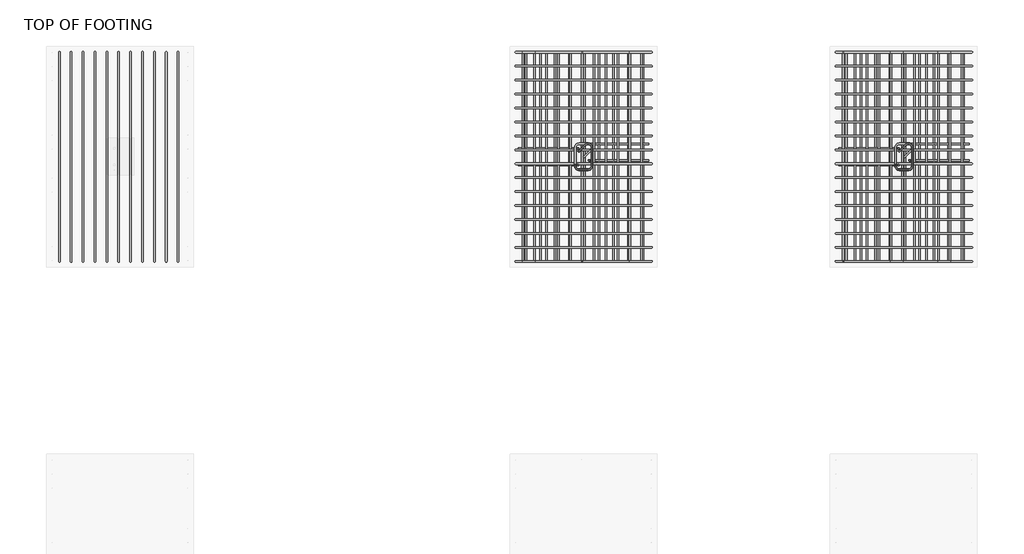
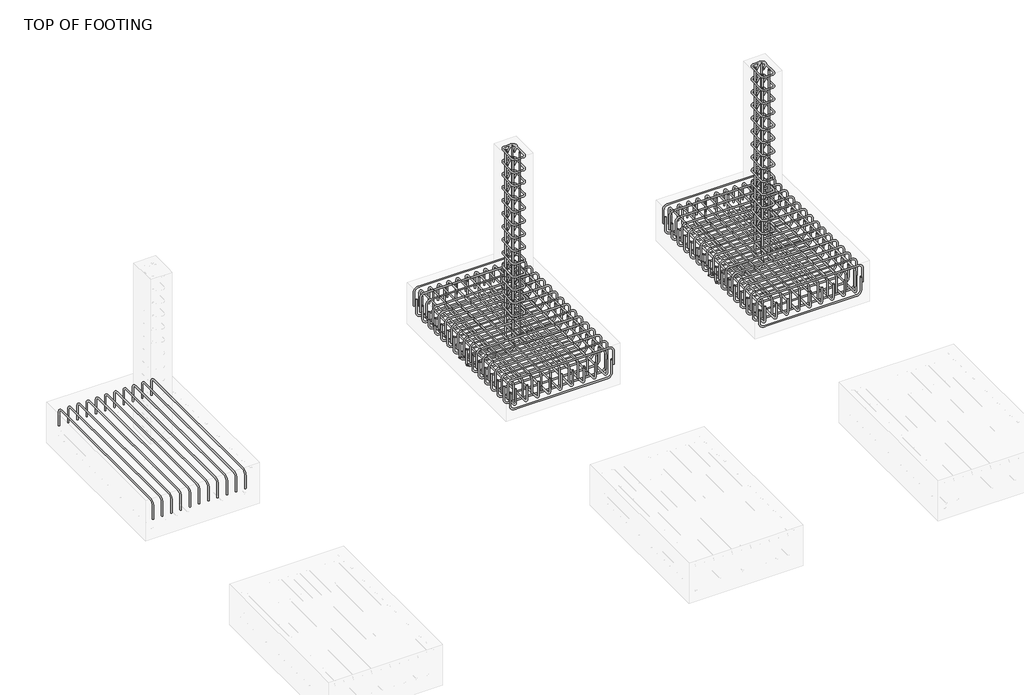
# One storey, part 8 of 8: 15 reinforcing bars.
"""IFC4 building model written with IfcOpenShell, lengths in millimetres."""

from ifc_helpers import new_model, si_unit, point, frame, origin, place, context, project, spatial, polyline, circle_curve, trimmed, segment, composite_curve, source, transform, mapped, element, save
from ifc_brep_helpers import swept_disk

model = new_model("IFC4")

# Units and contexts
model_context = context("Model", 3, world=origin())
ifc_project = project(units=[si_unit("LENGTHUNIT", "METRE", prefix="MILLI")], contexts=[model_context])

# Site, building, storey
site = spatial("IfcSite", under=ifc_project)
building = spatial("IfcBuilding", under=site)
storey = spatial("IfcBuildingStorey", under=building, Name="TOP OF FOOTING", Elevation=-1828.8)

# Reinforcing bars
placement = place(None, origin())
reinforcing_bar_shape = source(origin(), model_context, "Body", "SolidModel", [
    swept_disk(composite_curve([segment(polyline([(6846.0817577, 8966.4007933, -46.35), (6901.8253207, 9022.1443562, -46.35)]), True, "CONTINUOUS"), segment(trimmed(circle_curve(frame((6923.9931183, 8999.9765586, -46.35), z_axis=(0.0, 0.0, -1.0), x_axis=(-22.167797600000085, 22.167797600000995, 0.0)), 31.35), [point((6901.8253207, 9022.1443562, -46.35))], [point((6955.3431183, 8999.9765586, -46.35))], True, "CARTESIAN"), True, "CONTINUOUS"), segment(polyline([(6955.3431183, 8999.9765586, -46.35), (6955.3431183, 8850.5765586, -46.35)]), True, "CONTINUOUS"), segment(trimmed(circle_curve(frame((6923.9931183, 8850.5765586, -46.35), z_axis=(0.0, 0.0, -1.0), x_axis=(31.350000000000364, 0.0, 0.0)), 31.35), [point((6955.3431183, 8850.5765586, -46.35))], [point((6923.9931183, 8819.2265586, -46.35))], True, "CARTESIAN"), True, "CONTINUOUS"), segment(polyline([(6923.9931183, 8819.2265586, -46.35), (6850.7931183, 8819.2265586, -46.35)]), True, "CONTINUOUS"), segment(trimmed(circle_curve(frame((6850.7931183, 8850.5205096, -44.4761991), z_axis=(0.0, 0.05977036468717588, -0.9982121535551258), x_axis=(0.0, -31.29395100000147, -1.873800899999999)), 31.35), [point((6850.7931183, 8819.2265586, -46.35))], [point((6819.4431183, 8850.5205096, -44.4761991))], True, "CARTESIAN"), True, "CONTINUOUS"), segment(polyline([(6819.4431183, 8850.5205096, -44.4761991), (6819.4431183, 9000.0326076, -35.5238009)]), True, "CONTINUOUS"), segment(trimmed(circle_curve(frame((6850.7931183, 9000.0326076, -35.5238009), z_axis=(0.0, 0.05977036468717588, -0.9982121535551258), x_axis=(-31.350000000000364, 0.0, 0.0)), 31.35), [point((6819.4431183, 9000.0326076, -35.5238009))], [point((6850.7931183, 9031.3265586, -33.65))], True, "CARTESIAN"), True, "CONTINUOUS"), segment(polyline([(6850.7931183, 9031.3265586, -33.65), (6923.9931183, 9031.3265586, -33.65)]), True, "CONTINUOUS"), segment(trimmed(circle_curve(frame((6923.9931183, 8999.9765586, -33.65), z_axis=(0.0, 0.0, -1.0), x_axis=(0.0, 31.350000000000364, 0.0)), 31.35), [point((6923.9931183, 9031.3265586, -33.65))], [point((6946.1609159, 8977.808761, -33.65))], True, "CARTESIAN"), True, "CONTINUOUS"), segment(polyline([(6946.1609159, 8977.808761, -33.65), (6890.4173529, 8922.0651981, -33.65)]), True, "CONTINUOUS")], self_intersect=False), 6.35),
])
element("IfcReinforcingBar", 1, at=placement, inside=storey, context=model_context, shape_type="MappedRepresentation", body=[
    mapped(reinforcing_bar_shape, transform((0.0, 0.0, 0.0), x_axis=(1.0, 0.0, 0.0), y_axis=(0.0, 1.0, 0.0), z_axis=(0.0, 0.0, 1.0))),
    mapped(reinforcing_bar_shape, transform((0.0, 0.0, -144.675), x_axis=(1.0, 0.0, 0.0), y_axis=(0.0, 1.0, 0.0), z_axis=(0.0, 0.0, 1.0))),
    mapped(reinforcing_bar_shape, transform((0.0, 0.0, -289.35), x_axis=(1.0, 0.0, 0.0), y_axis=(0.0, 1.0, 0.0), z_axis=(0.0, 0.0, 1.0))),
    mapped(reinforcing_bar_shape, transform((0.0, 0.0, -434.025), x_axis=(1.0, 0.0, 0.0), y_axis=(0.0, 1.0, 0.0), z_axis=(0.0, 0.0, 1.0))),
    mapped(reinforcing_bar_shape, transform((0.0, 0.0, -578.7), x_axis=(1.0, 0.0, 0.0), y_axis=(0.0, 1.0, 0.0), z_axis=(0.0, 0.0, 1.0))),
    mapped(reinforcing_bar_shape, transform((0.0, 0.0, -723.375), x_axis=(1.0, 0.0, 0.0), y_axis=(0.0, 1.0, 0.0), z_axis=(0.0, 0.0, 1.0))),
    mapped(reinforcing_bar_shape, transform((0.0, 0.0, -868.05), x_axis=(1.0, 0.0, 0.0), y_axis=(0.0, 1.0, 0.0), z_axis=(0.0, 0.0, 1.0))),
    mapped(reinforcing_bar_shape, transform((0.0, 0.0, -1012.725), x_axis=(1.0, 0.0, 0.0), y_axis=(0.0, 1.0, 0.0), z_axis=(0.0, 0.0, 1.0))),
    mapped(reinforcing_bar_shape, transform((0.0, 0.0, -1157.4), x_axis=(1.0, 0.0, 0.0), y_axis=(0.0, 1.0, 0.0), z_axis=(0.0, 0.0, 1.0))),
    mapped(reinforcing_bar_shape, transform((0.0, 0.0, -1302.075), x_axis=(1.0, 0.0, 0.0), y_axis=(0.0, 1.0, 0.0), z_axis=(0.0, 0.0, 1.0))),
    mapped(reinforcing_bar_shape, transform((0.0, 0.0, -1446.75), x_axis=(1.0, 0.0, 0.0), y_axis=(0.0, 1.0, 0.0), z_axis=(0.0, 0.0, 1.0))),
    mapped(reinforcing_bar_shape, transform((0.0, 0.0, -1591.425), x_axis=(1.0, 0.0, 0.0), y_axis=(0.0, 1.0, 0.0), z_axis=(0.0, 0.0, 1.0))),
    mapped(reinforcing_bar_shape, transform((0.0, 0.0, -1736.1), x_axis=(1.0, 0.0, 0.0), y_axis=(0.0, 1.0, 0.0), z_axis=(0.0, 0.0, 1.0))),
])
reinforcing_bar_2_shape = source(origin(), model_context, "Body", "SolidModel", [
    swept_disk(composite_curve([segment(polyline([(7420.419602, 8895.4265586, -2177.1384798), (6979.2627797, 8895.4265586, -2177.1384798)]), True, "CONTINUOUS"), segment(trimmed(circle_curve(frame((6979.2627797, 8895.4265586, -2130.7884798), z_axis=(0.0, 1.0, 0.0), x_axis=(0.0, 0.0, -46.34999999999991)), 46.35), [point((6979.2627797, 8895.4265586, -2177.1384798))], [point((6932.9127797, 8895.4265586, -2130.7884798))], True, "CARTESIAN"), True, "CONTINUOUS"), segment(polyline([(6932.9127797, 8895.4265586, -2130.7884798), (6932.9127797, 8895.4265586, -40.0)]), True, "CONTINUOUS")], self_intersect=False), 6.35),
])
element("IfcReinforcingBar", 2, at=placement, inside=storey, context=model_context, shape_type="MappedRepresentation", body=[
    mapped(reinforcing_bar_2_shape, transform((0.0, 0.0, 0.0), x_axis=(1.0, 0.0, 0.0), y_axis=(0.0, 1.0, 0.0), z_axis=(0.0, 0.0, 1.0))),
    mapped(reinforcing_bar_2_shape, transform((0.0, 135.9, 0.0), x_axis=(1.0, 0.0, 0.0), y_axis=(0.0, 1.0, 0.0), z_axis=(0.0, 0.0, 1.0))),
])
reinforcing_bar_3_shape = source(origin(), model_context, "Body", "SolidModel", [
    swept_disk(composite_curve([segment(polyline([(6354.3666346, 8857.3265586, -2177.1384798), (6795.5234568, 8857.3265586, -2177.1384798)]), True, "CONTINUOUS"), segment(trimmed(circle_curve(frame((6795.5234568, 8857.3265586, -2130.7884798), z_axis=(0.0, -1.0, 0.0), x_axis=(0.0, 0.0, -46.34999999999991)), 46.35), [point((6795.5234568, 8857.3265586, -2177.1384798))], [point((6841.8734568, 8857.3265586, -2130.7884798))], True, "CARTESIAN"), True, "CONTINUOUS"), segment(polyline([(6841.8734568, 8857.3265586, -2130.7884798), (6841.8734568, 8857.3265586, -40.0)]), True, "CONTINUOUS")], self_intersect=False), 6.35),
])
element("IfcReinforcingBar", 3, at=placement, inside=storey, context=model_context, shape_type="MappedRepresentation", body=[
    mapped(reinforcing_bar_3_shape, transform((0.0, 0.0, 0.0), x_axis=(1.0, 0.0, 0.0), y_axis=(0.0, 1.0, 0.0), z_axis=(0.0, 0.0, 1.0))),
    mapped(reinforcing_bar_3_shape, transform((0.0, 135.9, 0.0), x_axis=(1.0, 0.0, 0.0), y_axis=(0.0, 1.0, 0.0), z_axis=(0.0, 0.0, 1.0))),
])
reinforcing_bar_4_shape = source(origin(), model_context, "Body", "SolidModel", [
    swept_disk(composite_curve([segment(polyline([(9462.2817577, 8966.4007933, -46.35), (9518.0253207, 9022.1443562, -46.35)]), True, "CONTINUOUS"), segment(trimmed(circle_curve(frame((9540.1931183, 8999.9765586, -46.35), z_axis=(0.0, 0.0, -1.0), x_axis=(-22.167797599999176, 22.167797600000995, 0.0)), 31.35), [point((9518.0253207, 9022.1443562, -46.35))], [point((9571.5431183, 8999.9765586, -46.35))], True, "CARTESIAN"), True, "CONTINUOUS"), segment(polyline([(9571.5431183, 8999.9765586, -46.35), (9571.5431183, 8850.5765586, -46.35)]), True, "CONTINUOUS"), segment(trimmed(circle_curve(frame((9540.1931183, 8850.5765586, -46.35), z_axis=(0.0, 0.0, -1.0), x_axis=(31.350000000000364, 0.0, 0.0)), 31.35), [point((9571.5431183, 8850.5765586, -46.35))], [point((9540.1931183, 8819.2265586, -46.35))], True, "CARTESIAN"), True, "CONTINUOUS"), segment(polyline([(9540.1931183, 8819.2265586, -46.35), (9466.9931183, 8819.2265586, -46.35)]), True, "CONTINUOUS"), segment(trimmed(circle_curve(frame((9466.9931183, 8850.5205096, -44.4761991), z_axis=(0.0, 0.05977036468717588, -0.9982121535551258), x_axis=(0.0, -31.29395100000147, -1.873800899999999)), 31.35), [point((9466.9931183, 8819.2265586, -46.35))], [point((9435.6431183, 8850.5205096, -44.4761991))], True, "CARTESIAN"), True, "CONTINUOUS"), segment(polyline([(9435.6431183, 8850.5205096, -44.4761991), (9435.6431183, 9000.0326076, -35.5238009)]), True, "CONTINUOUS"), segment(trimmed(circle_curve(frame((9466.9931183, 9000.0326076, -35.5238009), z_axis=(0.0, 0.05977036468717588, -0.9982121535551258), x_axis=(-31.350000000000364, 0.0, 0.0)), 31.35), [point((9435.6431183, 9000.0326076, -35.5238009))], [point((9466.9931183, 9031.3265586, -33.65))], True, "CARTESIAN"), True, "CONTINUOUS"), segment(polyline([(9466.9931183, 9031.3265586, -33.65), (9540.1931183, 9031.3265586, -33.65)]), True, "CONTINUOUS"), segment(trimmed(circle_curve(frame((9540.1931183, 8999.9765586, -33.65), z_axis=(0.0, 0.0, -1.0), x_axis=(0.0, 31.350000000000364, 0.0)), 31.35), [point((9540.1931183, 9031.3265586, -33.65))], [point((9562.3609159, 8977.808761, -33.65))], True, "CARTESIAN"), True, "CONTINUOUS"), segment(polyline([(9562.3609159, 8977.808761, -33.65), (9506.6173529, 8922.0651981, -33.65)]), True, "CONTINUOUS")], self_intersect=False), 6.35),
])
element("IfcReinforcingBar", 4, at=placement, inside=storey, context=model_context, shape_type="MappedRepresentation", body=[
    mapped(reinforcing_bar_4_shape, transform((0.0, 0.0, 0.0), x_axis=(1.0, 0.0, 0.0), y_axis=(0.0, 1.0, 0.0), z_axis=(0.0, 0.0, 1.0))),
    mapped(reinforcing_bar_4_shape, transform((0.0, 0.0, -144.675), x_axis=(1.0, 0.0, 0.0), y_axis=(0.0, 1.0, 0.0), z_axis=(0.0, 0.0, 1.0))),
    mapped(reinforcing_bar_4_shape, transform((0.0, 0.0, -289.35), x_axis=(1.0, 0.0, 0.0), y_axis=(0.0, 1.0, 0.0), z_axis=(0.0, 0.0, 1.0))),
    mapped(reinforcing_bar_4_shape, transform((0.0, 0.0, -434.025), x_axis=(1.0, 0.0, 0.0), y_axis=(0.0, 1.0, 0.0), z_axis=(0.0, 0.0, 1.0))),
    mapped(reinforcing_bar_4_shape, transform((0.0, 0.0, -578.7), x_axis=(1.0, 0.0, 0.0), y_axis=(0.0, 1.0, 0.0), z_axis=(0.0, 0.0, 1.0))),
    mapped(reinforcing_bar_4_shape, transform((0.0, 0.0, -723.375), x_axis=(1.0, 0.0, 0.0), y_axis=(0.0, 1.0, 0.0), z_axis=(0.0, 0.0, 1.0))),
    mapped(reinforcing_bar_4_shape, transform((0.0, 0.0, -868.05), x_axis=(1.0, 0.0, 0.0), y_axis=(0.0, 1.0, 0.0), z_axis=(0.0, 0.0, 1.0))),
    mapped(reinforcing_bar_4_shape, transform((0.0, 0.0, -1012.725), x_axis=(1.0, 0.0, 0.0), y_axis=(0.0, 1.0, 0.0), z_axis=(0.0, 0.0, 1.0))),
    mapped(reinforcing_bar_4_shape, transform((0.0, 0.0, -1157.4), x_axis=(1.0, 0.0, 0.0), y_axis=(0.0, 1.0, 0.0), z_axis=(0.0, 0.0, 1.0))),
    mapped(reinforcing_bar_4_shape, transform((0.0, 0.0, -1302.075), x_axis=(1.0, 0.0, 0.0), y_axis=(0.0, 1.0, 0.0), z_axis=(0.0, 0.0, 1.0))),
    mapped(reinforcing_bar_4_shape, transform((0.0, 0.0, -1446.75), x_axis=(1.0, 0.0, 0.0), y_axis=(0.0, 1.0, 0.0), z_axis=(0.0, 0.0, 1.0))),
    mapped(reinforcing_bar_4_shape, transform((0.0, 0.0, -1591.425), x_axis=(1.0, 0.0, 0.0), y_axis=(0.0, 1.0, 0.0), z_axis=(0.0, 0.0, 1.0))),
    mapped(reinforcing_bar_4_shape, transform((0.0, 0.0, -1736.1), x_axis=(1.0, 0.0, 0.0), y_axis=(0.0, 1.0, 0.0), z_axis=(0.0, 0.0, 1.0))),
])
reinforcing_bar_5_shape = source(origin(), model_context, "Body", "SolidModel", [
    swept_disk(composite_curve([segment(polyline([(10036.619602, 8895.4265586, -2177.1384798), (9595.4627797, 8895.4265586, -2177.1384798)]), True, "CONTINUOUS"), segment(trimmed(circle_curve(frame((9595.4627797, 8895.4265586, -2130.7884798), z_axis=(0.0, 1.0, 0.0), x_axis=(0.0, 0.0, -46.34999999999991)), 46.35), [point((9595.4627797, 8895.4265586, -2177.1384798))], [point((9549.1127797, 8895.4265586, -2130.7884798))], True, "CARTESIAN"), True, "CONTINUOUS"), segment(polyline([(9549.1127797, 8895.4265586, -2130.7884798), (9549.1127797, 8895.4265586, -40.0)]), True, "CONTINUOUS")], self_intersect=False), 6.35),
])
element("IfcReinforcingBar", 5, at=placement, inside=storey, context=model_context, shape_type="MappedRepresentation", body=[
    mapped(reinforcing_bar_5_shape, transform((0.0, 0.0, 0.0), x_axis=(1.0, 0.0, 0.0), y_axis=(0.0, 1.0, 0.0), z_axis=(0.0, 0.0, 1.0))),
    mapped(reinforcing_bar_5_shape, transform((0.0, 135.9, 0.0), x_axis=(1.0, 0.0, 0.0), y_axis=(0.0, 1.0, 0.0), z_axis=(0.0, 0.0, 1.0))),
])
reinforcing_bar_6_shape = source(origin(), model_context, "Body", "SolidModel", [
    swept_disk(composite_curve([segment(polyline([(8970.5666346, 8857.3265586, -2177.1384798), (9411.7234568, 8857.3265586, -2177.1384798)]), True, "CONTINUOUS"), segment(trimmed(circle_curve(frame((9411.7234568, 8857.3265586, -2130.7884798), z_axis=(0.0, -1.0, 0.0), x_axis=(0.0, 0.0, -46.34999999999991)), 46.35), [point((9411.7234568, 8857.3265586, -2177.1384798))], [point((9458.0734568, 8857.3265586, -2130.7884798))], True, "CARTESIAN"), True, "CONTINUOUS"), segment(polyline([(9458.0734568, 8857.3265586, -2130.7884798), (9458.0734568, 8857.3265586, -40.0)]), True, "CONTINUOUS")], self_intersect=False), 6.35),
])
element("IfcReinforcingBar", 6, at=placement, inside=storey, context=model_context, shape_type="MappedRepresentation", body=[
    mapped(reinforcing_bar_6_shape, transform((0.0, 0.0, 0.0), x_axis=(1.0, 0.0, 0.0), y_axis=(0.0, 1.0, 0.0), z_axis=(0.0, 0.0, 1.0))),
    mapped(reinforcing_bar_6_shape, transform((0.0, 135.9, 0.0), x_axis=(1.0, 0.0, 0.0), y_axis=(0.0, 1.0, 0.0), z_axis=(0.0, 0.0, 1.0))),
])
reinforcing_bar_7_shape = source(origin(), model_context, "Body", "SolidModel", [
    swept_disk(composite_curve([segment(polyline([(3577.1331701, 9778.9265586, -2094.8977257), (3577.1331701, 9778.9265586, -1947.5977257)]), True, "CONTINUOUS"), segment(trimmed(circle_curve(frame((3577.1331701, 9732.5765586, -1947.5977257), z_axis=(1.0, 0.0, 0.0), x_axis=(0.0, 46.350000000000364, 0.0)), 46.35), [point((3577.1331701, 9778.9265586, -1947.5977257))], [point((3577.1331701, 9732.5765586, -1901.2477257))], True, "CARTESIAN"), True, "CONTINUOUS"), segment(polyline([(3577.1331701, 9732.5765586, -1901.2477257), (3577.1331701, 8117.9765586, -1901.2477257)]), True, "CONTINUOUS"), segment(trimmed(circle_curve(frame((3577.1331701, 8117.9765586, -1947.5977257), z_axis=(1.0, 0.0, 0.0), x_axis=(0.0, 0.0, 46.34999999999991)), 46.35), [point((3577.1331701, 8117.9765586, -1901.2477257))], [point((3577.1331701, 8071.6265586, -1947.5977257))], True, "CARTESIAN"), True, "CONTINUOUS"), segment(polyline([(3577.1331701, 8071.6265586, -1947.5977257), (3577.1331701, 8071.6265586, -2094.8977257)]), True, "CONTINUOUS")], self_intersect=False), 6.35),
])
element("IfcReinforcingBar", 7, at=placement, inside=storey, context=model_context, shape_type="MappedRepresentation", body=[
    mapped(reinforcing_bar_7_shape, transform((0.0, 0.0, 0.0), x_axis=(1.0, 0.0, 0.0), y_axis=(0.0, 1.0, 0.0), z_axis=(0.0, 0.0, 1.0))),
    mapped(reinforcing_bar_7_shape, transform((-97.0050815, 0.0, 0.0), x_axis=(1.0, 0.0, 0.0), y_axis=(0.0, 1.0, 0.0), z_axis=(0.0, 0.0, 1.0))),
    mapped(reinforcing_bar_7_shape, transform((-194.0101631, 0.0, 0.0), x_axis=(1.0, 0.0, 0.0), y_axis=(0.0, 1.0, 0.0), z_axis=(0.0, 0.0, 1.0))),
    mapped(reinforcing_bar_7_shape, transform((-291.0152446, 0.0, 0.0), x_axis=(1.0, 0.0, 0.0), y_axis=(0.0, 1.0, 0.0), z_axis=(0.0, 0.0, 1.0))),
    mapped(reinforcing_bar_7_shape, transform((-388.0203261, 0.0, 0.0), x_axis=(1.0, 0.0, 0.0), y_axis=(0.0, 1.0, 0.0), z_axis=(0.0, 0.0, 1.0))),
    mapped(reinforcing_bar_7_shape, transform((-485.0254076, 0.0, 0.0), x_axis=(1.0, 0.0, 0.0), y_axis=(0.0, 1.0, 0.0), z_axis=(0.0, 0.0, 1.0))),
    mapped(reinforcing_bar_7_shape, transform((-582.0304892, 0.0, 0.0), x_axis=(1.0, 0.0, 0.0), y_axis=(0.0, 1.0, 0.0), z_axis=(0.0, 0.0, 1.0))),
    mapped(reinforcing_bar_7_shape, transform((-679.0355707, 0.0, 0.0), x_axis=(1.0, 0.0, 0.0), y_axis=(0.0, 1.0, 0.0), z_axis=(0.0, 0.0, 1.0))),
    mapped(reinforcing_bar_7_shape, transform((-776.0406522, 0.0, 0.0), x_axis=(1.0, 0.0, 0.0), y_axis=(0.0, 1.0, 0.0), z_axis=(0.0, 0.0, 1.0))),
    mapped(reinforcing_bar_7_shape, transform((-873.0457338, 0.0, 0.0), x_axis=(1.0, 0.0, 0.0), y_axis=(0.0, 1.0, 0.0), z_axis=(0.0, 0.0, 1.0))),
    mapped(reinforcing_bar_7_shape, transform((-970.0508153, 0.0, 0.0), x_axis=(1.0, 0.0, 0.0), y_axis=(0.0, 1.0, 0.0), z_axis=(0.0, 0.0, 1.0))),
])
reinforcing_bar_8_shape = source(origin(), model_context, "Body", "SolidModel", [
    swept_disk(composite_curve([segment(polyline([(7421.6426771, 9778.9265586, -2008.2544267), (7421.6426771, 9778.9265586, -2155.5544267)]), True, "CONTINUOUS"), segment(trimmed(circle_curve(frame((7375.2926771, 9778.9265586, -2155.5544267), z_axis=(0.0, 1.0, 0.0), x_axis=(46.349999999999454, 0.0, 0.0)), 46.35), [point((7421.6426771, 9778.9265586, -2155.5544267))], [point((7375.2926771, 9778.9265586, -2201.9044267))], True, "CARTESIAN"), True, "CONTINUOUS"), segment(polyline([(7375.2926771, 9778.9265586, -2201.9044267), (6404.2766408, 9778.9265586, -2201.9044267)]), True, "CONTINUOUS"), segment(trimmed(circle_curve(frame((6404.2766408, 9778.9265586, -2155.5544267), z_axis=(0.0, 1.0, 0.0), x_axis=(0.0, 0.0, -46.34999999999991)), 46.35), [point((6404.2766408, 9778.9265586, -2201.9044267))], [point((6357.9266408, 9778.9265586, -2155.5544267))], True, "CARTESIAN"), True, "CONTINUOUS"), segment(polyline([(6357.9266408, 9778.9265586, -2155.5544267), (6357.9266408, 9778.9265586, -2008.2544267)]), True, "CONTINUOUS")], self_intersect=False), 6.35),
])
element("IfcReinforcingBar", 8, at=placement, inside=storey, context=model_context, shape_type="MappedRepresentation", body=[
    mapped(reinforcing_bar_8_shape, transform((0.0, 0.0, 0.0), x_axis=(1.0, 0.0, 0.0), y_axis=(0.0, 1.0, 0.0), z_axis=(0.0, 0.0, 1.0))),
    mapped(reinforcing_bar_8_shape, transform((0.0, -113.82, 0.0), x_axis=(1.0, 0.0, 0.0), y_axis=(0.0, 1.0, 0.0), z_axis=(0.0, 0.0, 1.0))),
    mapped(reinforcing_bar_8_shape, transform((0.0, -227.64, 0.0), x_axis=(1.0, 0.0, 0.0), y_axis=(0.0, 1.0, 0.0), z_axis=(0.0, 0.0, 1.0))),
    mapped(reinforcing_bar_8_shape, transform((0.0, -341.46, 0.0), x_axis=(1.0, 0.0, 0.0), y_axis=(0.0, 1.0, 0.0), z_axis=(0.0, 0.0, 1.0))),
    mapped(reinforcing_bar_8_shape, transform((0.0, -455.28, 0.0), x_axis=(1.0, 0.0, 0.0), y_axis=(0.0, 1.0, 0.0), z_axis=(0.0, 0.0, 1.0))),
    mapped(reinforcing_bar_8_shape, transform((0.0, -569.1, 0.0), x_axis=(1.0, 0.0, 0.0), y_axis=(0.0, 1.0, 0.0), z_axis=(0.0, 0.0, 1.0))),
    mapped(reinforcing_bar_8_shape, transform((0.0, -682.92, 0.0), x_axis=(1.0, 0.0, 0.0), y_axis=(0.0, 1.0, 0.0), z_axis=(0.0, 0.0, 1.0))),
    mapped(reinforcing_bar_8_shape, transform((0.0, -796.74, 0.0), x_axis=(1.0, 0.0, 0.0), y_axis=(0.0, 1.0, 0.0), z_axis=(0.0, 0.0, 1.0))),
    mapped(reinforcing_bar_8_shape, transform((0.0, -910.56, 0.0), x_axis=(1.0, 0.0, 0.0), y_axis=(0.0, 1.0, 0.0), z_axis=(0.0, 0.0, 1.0))),
    mapped(reinforcing_bar_8_shape, transform((0.0, -1024.38, 0.0), x_axis=(1.0, 0.0, 0.0), y_axis=(0.0, 1.0, 0.0), z_axis=(0.0, 0.0, 1.0))),
    mapped(reinforcing_bar_8_shape, transform((0.0, -1138.2, 0.0), x_axis=(1.0, 0.0, 0.0), y_axis=(0.0, 1.0, 0.0), z_axis=(0.0, 0.0, 1.0))),
    mapped(reinforcing_bar_8_shape, transform((0.0, -1252.02, 0.0), x_axis=(1.0, 0.0, 0.0), y_axis=(0.0, 1.0, 0.0), z_axis=(0.0, 0.0, 1.0))),
    mapped(reinforcing_bar_8_shape, transform((0.0, -1365.84, 0.0), x_axis=(1.0, 0.0, 0.0), y_axis=(0.0, 1.0, 0.0), z_axis=(0.0, 0.0, 1.0))),
    mapped(reinforcing_bar_8_shape, transform((0.0, -1479.66, 0.0), x_axis=(1.0, 0.0, 0.0), y_axis=(0.0, 1.0, 0.0), z_axis=(0.0, 0.0, 1.0))),
    mapped(reinforcing_bar_8_shape, transform((0.0, -1593.48, 0.0), x_axis=(1.0, 0.0, 0.0), y_axis=(0.0, 1.0, 0.0), z_axis=(0.0, 0.0, 1.0))),
    mapped(reinforcing_bar_8_shape, transform((0.0, -1707.3, 0.0), x_axis=(1.0, 0.0, 0.0), y_axis=(0.0, 1.0, 0.0), z_axis=(0.0, 0.0, 1.0))),
])
reinforcing_bar_9_shape = source(origin(), model_context, "Body", "SolidModel", [
    swept_disk(composite_curve([segment(polyline([(6333.7431183, 9778.9265586, -2068.8), (6333.7431183, 9778.9265586, -1921.5)]), True, "CONTINUOUS"), segment(trimmed(circle_curve(frame((6380.0931183, 9778.9265586, -1921.5), z_axis=(0.0, 1.0, 0.0), x_axis=(-46.350000000000364, 0.0, 0.0)), 46.35), [point((6333.7431183, 9778.9265586, -1921.5))], [point((6380.0931183, 9778.9265586, -1875.15))], True, "CARTESIAN"), True, "CONTINUOUS"), segment(polyline([(6380.0931183, 9778.9265586, -1875.15), (7394.6931183, 9778.9265586, -1875.15)]), True, "CONTINUOUS"), segment(trimmed(circle_curve(frame((7394.6931183, 9778.9265586, -1921.5), z_axis=(0.0, 1.0, 0.0), x_axis=(0.0, 0.0, 46.34999999999991)), 46.35), [point((7394.6931183, 9778.9265586, -1875.15))], [point((7441.0431183, 9778.9265586, -1921.5))], True, "CARTESIAN"), True, "CONTINUOUS"), segment(polyline([(7441.0431183, 9778.9265586, -1921.5), (7441.0431183, 9778.9265586, -2068.8)]), True, "CONTINUOUS")], self_intersect=False), 6.35),
])
element("IfcReinforcingBar", 9, at=placement, inside=storey, context=model_context, shape_type="MappedRepresentation", body=[
    mapped(reinforcing_bar_9_shape, transform((0.0, 0.0, 0.0), x_axis=(1.0, 0.0, 0.0), y_axis=(0.0, 1.0, 0.0), z_axis=(0.0, 0.0, 1.0))),
    mapped(reinforcing_bar_9_shape, transform((0.0, -113.82, 0.0), x_axis=(1.0, 0.0, 0.0), y_axis=(0.0, 1.0, 0.0), z_axis=(0.0, 0.0, 1.0))),
    mapped(reinforcing_bar_9_shape, transform((0.0, -227.64, 0.0), x_axis=(1.0, 0.0, 0.0), y_axis=(0.0, 1.0, 0.0), z_axis=(0.0, 0.0, 1.0))),
    mapped(reinforcing_bar_9_shape, transform((0.0, -341.46, 0.0), x_axis=(1.0, 0.0, 0.0), y_axis=(0.0, 1.0, 0.0), z_axis=(0.0, 0.0, 1.0))),
    mapped(reinforcing_bar_9_shape, transform((0.0, -455.28, 0.0), x_axis=(1.0, 0.0, 0.0), y_axis=(0.0, 1.0, 0.0), z_axis=(0.0, 0.0, 1.0))),
    mapped(reinforcing_bar_9_shape, transform((0.0, -569.1, 0.0), x_axis=(1.0, 0.0, 0.0), y_axis=(0.0, 1.0, 0.0), z_axis=(0.0, 0.0, 1.0))),
    mapped(reinforcing_bar_9_shape, transform((0.0, -682.92, 0.0), x_axis=(1.0, 0.0, 0.0), y_axis=(0.0, 1.0, 0.0), z_axis=(0.0, 0.0, 1.0))),
    mapped(reinforcing_bar_9_shape, transform((0.0, -796.74, 0.0), x_axis=(1.0, 0.0, 0.0), y_axis=(0.0, 1.0, 0.0), z_axis=(0.0, 0.0, 1.0))),
    mapped(reinforcing_bar_9_shape, transform((0.0, -910.56, 0.0), x_axis=(1.0, 0.0, 0.0), y_axis=(0.0, 1.0, 0.0), z_axis=(0.0, 0.0, 1.0))),
    mapped(reinforcing_bar_9_shape, transform((0.0, -1024.38, 0.0), x_axis=(1.0, 0.0, 0.0), y_axis=(0.0, 1.0, 0.0), z_axis=(0.0, 0.0, 1.0))),
    mapped(reinforcing_bar_9_shape, transform((0.0, -1138.2, 0.0), x_axis=(1.0, 0.0, 0.0), y_axis=(0.0, 1.0, 0.0), z_axis=(0.0, 0.0, 1.0))),
    mapped(reinforcing_bar_9_shape, transform((0.0, -1252.02, 0.0), x_axis=(1.0, 0.0, 0.0), y_axis=(0.0, 1.0, 0.0), z_axis=(0.0, 0.0, 1.0))),
    mapped(reinforcing_bar_9_shape, transform((0.0, -1365.84, 0.0), x_axis=(1.0, 0.0, 0.0), y_axis=(0.0, 1.0, 0.0), z_axis=(0.0, 0.0, 1.0))),
    mapped(reinforcing_bar_9_shape, transform((0.0, -1479.66, 0.0), x_axis=(1.0, 0.0, 0.0), y_axis=(0.0, 1.0, 0.0), z_axis=(0.0, 0.0, 1.0))),
    mapped(reinforcing_bar_9_shape, transform((0.0, -1593.48, 0.0), x_axis=(1.0, 0.0, 0.0), y_axis=(0.0, 1.0, 0.0), z_axis=(0.0, 0.0, 1.0))),
    mapped(reinforcing_bar_9_shape, transform((0.0, -1707.3, 0.0), x_axis=(1.0, 0.0, 0.0), y_axis=(0.0, 1.0, 0.0), z_axis=(0.0, 0.0, 1.0))),
])
reinforcing_bar_10_shape = source(origin(), model_context, "Body", "SolidModel", [
    swept_disk(composite_curve([segment(polyline([(6415.9651697, 9778.9265586, -1986.9111268), (6415.9651697, 9778.9265586, -2134.2111268)]), True, "CONTINUOUS"), segment(trimmed(circle_curve(frame((6415.9651697, 9732.5765586, -2134.2111268), z_axis=(-1.0, 0.0, 0.0), x_axis=(0.0, 46.350000000000364, 0.0)), 46.35), [point((6415.9651697, 9778.9265586, -2134.2111268))], [point((6415.9651697, 9732.5765586, -2180.5611268))], True, "CARTESIAN"), True, "CONTINUOUS"), segment(polyline([(6415.9651697, 9732.5765586, -2180.5611268), (6415.9651697, 8117.9765586, -2180.5611268)]), True, "CONTINUOUS"), segment(trimmed(circle_curve(frame((6415.9651697, 8117.9765586, -2134.2111268), z_axis=(-1.0, 0.0, 0.0), x_axis=(0.0, 0.0, -46.34999999999991)), 46.35), [point((6415.9651697, 8117.9765586, -2180.5611268))], [point((6415.9651697, 8071.6265586, -2134.2111268))], True, "CARTESIAN"), True, "CONTINUOUS"), segment(polyline([(6415.9651697, 8071.6265586, -2134.2111268), (6415.9651697, 8071.6265586, -1986.9111268)]), True, "CONTINUOUS")], self_intersect=False), 6.35),
])
element("IfcReinforcingBar", 10, at=placement, inside=storey, context=model_context, shape_type="MappedRepresentation", body=[
    mapped(reinforcing_bar_10_shape, transform((0.0, 0.0, 0.0), x_axis=(1.0, 0.0, 0.0), y_axis=(0.0, 1.0, 0.0), z_axis=(0.0, 0.0, 1.0))),
    mapped(reinforcing_bar_10_shape, transform((119.5564677, 0.0, 0.0), x_axis=(1.0, 0.0, 0.0), y_axis=(0.0, 1.0, 0.0), z_axis=(0.0, 0.0, 1.0))),
    mapped(reinforcing_bar_10_shape, transform((239.1129355, 0.0, 0.0), x_axis=(1.0, 0.0, 0.0), y_axis=(0.0, 1.0, 0.0), z_axis=(0.0, 0.0, 1.0))),
    mapped(reinforcing_bar_10_shape, transform((358.6694032, 0.0, 0.0), x_axis=(1.0, 0.0, 0.0), y_axis=(0.0, 1.0, 0.0), z_axis=(0.0, 0.0, 1.0))),
    mapped(reinforcing_bar_10_shape, transform((478.2258709, 0.0, 0.0), x_axis=(1.0, 0.0, 0.0), y_axis=(0.0, 1.0, 0.0), z_axis=(0.0, 0.0, 1.0))),
    mapped(reinforcing_bar_10_shape, transform((597.7823387, 0.0, 0.0), x_axis=(1.0, 0.0, 0.0), y_axis=(0.0, 1.0, 0.0), z_axis=(0.0, 0.0, 1.0))),
    mapped(reinforcing_bar_10_shape, transform((717.3388064, 0.0, 0.0), x_axis=(1.0, 0.0, 0.0), y_axis=(0.0, 1.0, 0.0), z_axis=(0.0, 0.0, 1.0))),
    mapped(reinforcing_bar_10_shape, transform((836.8952741, 0.0, 0.0), x_axis=(1.0, 0.0, 0.0), y_axis=(0.0, 1.0, 0.0), z_axis=(0.0, 0.0, 1.0))),
    mapped(reinforcing_bar_10_shape, transform((956.4517419, 0.0, 0.0), x_axis=(1.0, 0.0, 0.0), y_axis=(0.0, 1.0, 0.0), z_axis=(0.0, 0.0, 1.0))),
])
reinforcing_bar_11_shape = source(origin(), model_context, "Body", "SolidModel", [
    swept_disk(composite_curve([segment(polyline([(7361.7331701, 9778.9265586, -2094.8977257), (7361.7331701, 9778.9265586, -1947.5977257)]), True, "CONTINUOUS"), segment(trimmed(circle_curve(frame((7361.7331701, 9732.5765586, -1947.5977257), z_axis=(1.0, 0.0, 0.0), x_axis=(0.0, 46.350000000000364, 0.0)), 46.35), [point((7361.7331701, 9778.9265586, -1947.5977257))], [point((7361.7331701, 9732.5765586, -1901.2477257))], True, "CARTESIAN"), True, "CONTINUOUS"), segment(polyline([(7361.7331701, 9732.5765586, -1901.2477257), (7361.7331701, 8117.9765586, -1901.2477257)]), True, "CONTINUOUS"), segment(trimmed(circle_curve(frame((7361.7331701, 8117.9765586, -1947.5977257), z_axis=(1.0, 0.0, 0.0), x_axis=(0.0, 0.0, 46.34999999999991)), 46.35), [point((7361.7331701, 8117.9765586, -1901.2477257))], [point((7361.7331701, 8071.6265586, -1947.5977257))], True, "CARTESIAN"), True, "CONTINUOUS"), segment(polyline([(7361.7331701, 8071.6265586, -1947.5977257), (7361.7331701, 8071.6265586, -2094.8977257)]), True, "CONTINUOUS")], self_intersect=False), 6.35),
])
element("IfcReinforcingBar", 11, at=placement, inside=storey, context=model_context, shape_type="MappedRepresentation", body=[
    mapped(reinforcing_bar_11_shape, transform((0.0, 0.0, 0.0), x_axis=(1.0, 0.0, 0.0), y_axis=(0.0, 1.0, 0.0), z_axis=(0.0, 0.0, 1.0))),
    mapped(reinforcing_bar_11_shape, transform((-97.0050815, 0.0, 0.0), x_axis=(1.0, 0.0, 0.0), y_axis=(0.0, 1.0, 0.0), z_axis=(0.0, 0.0, 1.0))),
    mapped(reinforcing_bar_11_shape, transform((-194.0101631, 0.0, 0.0), x_axis=(1.0, 0.0, 0.0), y_axis=(0.0, 1.0, 0.0), z_axis=(0.0, 0.0, 1.0))),
    mapped(reinforcing_bar_11_shape, transform((-291.0152446, 0.0, 0.0), x_axis=(1.0, 0.0, 0.0), y_axis=(0.0, 1.0, 0.0), z_axis=(0.0, 0.0, 1.0))),
    mapped(reinforcing_bar_11_shape, transform((-388.0203261, 0.0, 0.0), x_axis=(1.0, 0.0, 0.0), y_axis=(0.0, 1.0, 0.0), z_axis=(0.0, 0.0, 1.0))),
    mapped(reinforcing_bar_11_shape, transform((-485.0254076, 0.0, 0.0), x_axis=(1.0, 0.0, 0.0), y_axis=(0.0, 1.0, 0.0), z_axis=(0.0, 0.0, 1.0))),
    mapped(reinforcing_bar_11_shape, transform((-582.0304892, 0.0, 0.0), x_axis=(1.0, 0.0, 0.0), y_axis=(0.0, 1.0, 0.0), z_axis=(0.0, 0.0, 1.0))),
    mapped(reinforcing_bar_11_shape, transform((-679.0355707, 0.0, 0.0), x_axis=(1.0, 0.0, 0.0), y_axis=(0.0, 1.0, 0.0), z_axis=(0.0, 0.0, 1.0))),
    mapped(reinforcing_bar_11_shape, transform((-776.0406522, 0.0, 0.0), x_axis=(1.0, 0.0, 0.0), y_axis=(0.0, 1.0, 0.0), z_axis=(0.0, 0.0, 1.0))),
    mapped(reinforcing_bar_11_shape, transform((-873.0457338, 0.0, 0.0), x_axis=(1.0, 0.0, 0.0), y_axis=(0.0, 1.0, 0.0), z_axis=(0.0, 0.0, 1.0))),
    mapped(reinforcing_bar_11_shape, transform((-970.0508153, 0.0, 0.0), x_axis=(1.0, 0.0, 0.0), y_axis=(0.0, 1.0, 0.0), z_axis=(0.0, 0.0, 1.0))),
])
reinforcing_bar_12_shape = source(origin(), model_context, "Body", "SolidModel", [
    swept_disk(composite_curve([segment(polyline([(10037.8426771, 9778.9265586, -2008.2544267), (10037.8426771, 9778.9265586, -2155.5544267)]), True, "CONTINUOUS"), segment(trimmed(circle_curve(frame((9991.4926771, 9778.9265586, -2155.5544267), z_axis=(0.0, 1.0, 0.0), x_axis=(46.350000000000364, 0.0, 0.0)), 46.35), [point((10037.8426771, 9778.9265586, -2155.5544267))], [point((9991.4926771, 9778.9265586, -2201.9044267))], True, "CARTESIAN"), True, "CONTINUOUS"), segment(polyline([(9991.4926771, 9778.9265586, -2201.9044267), (9020.4766408, 9778.9265586, -2201.9044267)]), True, "CONTINUOUS"), segment(trimmed(circle_curve(frame((9020.4766408, 9778.9265586, -2155.5544267), z_axis=(0.0, 1.0, 0.0), x_axis=(0.0, 0.0, -46.34999999999991)), 46.35), [point((9020.4766408, 9778.9265586, -2201.9044267))], [point((8974.1266408, 9778.9265586, -2155.5544267))], True, "CARTESIAN"), True, "CONTINUOUS"), segment(polyline([(8974.1266408, 9778.9265586, -2155.5544267), (8974.1266408, 9778.9265586, -2008.2544267)]), True, "CONTINUOUS")], self_intersect=False), 6.35),
])
element("IfcReinforcingBar", 12, at=placement, inside=storey, context=model_context, shape_type="MappedRepresentation", body=[
    mapped(reinforcing_bar_12_shape, transform((0.0, 0.0, 0.0), x_axis=(1.0, 0.0, 0.0), y_axis=(0.0, 1.0, 0.0), z_axis=(0.0, 0.0, 1.0))),
    mapped(reinforcing_bar_12_shape, transform((0.0, -113.82, 0.0), x_axis=(1.0, 0.0, 0.0), y_axis=(0.0, 1.0, 0.0), z_axis=(0.0, 0.0, 1.0))),
    mapped(reinforcing_bar_12_shape, transform((0.0, -227.64, 0.0), x_axis=(1.0, 0.0, 0.0), y_axis=(0.0, 1.0, 0.0), z_axis=(0.0, 0.0, 1.0))),
    mapped(reinforcing_bar_12_shape, transform((0.0, -341.46, 0.0), x_axis=(1.0, 0.0, 0.0), y_axis=(0.0, 1.0, 0.0), z_axis=(0.0, 0.0, 1.0))),
    mapped(reinforcing_bar_12_shape, transform((0.0, -455.28, 0.0), x_axis=(1.0, 0.0, 0.0), y_axis=(0.0, 1.0, 0.0), z_axis=(0.0, 0.0, 1.0))),
    mapped(reinforcing_bar_12_shape, transform((0.0, -569.1, 0.0), x_axis=(1.0, 0.0, 0.0), y_axis=(0.0, 1.0, 0.0), z_axis=(0.0, 0.0, 1.0))),
    mapped(reinforcing_bar_12_shape, transform((0.0, -682.92, 0.0), x_axis=(1.0, 0.0, 0.0), y_axis=(0.0, 1.0, 0.0), z_axis=(0.0, 0.0, 1.0))),
    mapped(reinforcing_bar_12_shape, transform((0.0, -796.74, 0.0), x_axis=(1.0, 0.0, 0.0), y_axis=(0.0, 1.0, 0.0), z_axis=(0.0, 0.0, 1.0))),
    mapped(reinforcing_bar_12_shape, transform((0.0, -910.56, 0.0), x_axis=(1.0, 0.0, 0.0), y_axis=(0.0, 1.0, 0.0), z_axis=(0.0, 0.0, 1.0))),
    mapped(reinforcing_bar_12_shape, transform((0.0, -1024.38, 0.0), x_axis=(1.0, 0.0, 0.0), y_axis=(0.0, 1.0, 0.0), z_axis=(0.0, 0.0, 1.0))),
    mapped(reinforcing_bar_12_shape, transform((0.0, -1138.2, 0.0), x_axis=(1.0, 0.0, 0.0), y_axis=(0.0, 1.0, 0.0), z_axis=(0.0, 0.0, 1.0))),
    mapped(reinforcing_bar_12_shape, transform((0.0, -1252.02, 0.0), x_axis=(1.0, 0.0, 0.0), y_axis=(0.0, 1.0, 0.0), z_axis=(0.0, 0.0, 1.0))),
    mapped(reinforcing_bar_12_shape, transform((0.0, -1365.84, 0.0), x_axis=(1.0, 0.0, 0.0), y_axis=(0.0, 1.0, 0.0), z_axis=(0.0, 0.0, 1.0))),
    mapped(reinforcing_bar_12_shape, transform((0.0, -1479.66, 0.0), x_axis=(1.0, 0.0, 0.0), y_axis=(0.0, 1.0, 0.0), z_axis=(0.0, 0.0, 1.0))),
    mapped(reinforcing_bar_12_shape, transform((0.0, -1593.48, 0.0), x_axis=(1.0, 0.0, 0.0), y_axis=(0.0, 1.0, 0.0), z_axis=(0.0, 0.0, 1.0))),
    mapped(reinforcing_bar_12_shape, transform((0.0, -1707.3, 0.0), x_axis=(1.0, 0.0, 0.0), y_axis=(0.0, 1.0, 0.0), z_axis=(0.0, 0.0, 1.0))),
])
reinforcing_bar_13_shape = source(origin(), model_context, "Body", "SolidModel", [
    swept_disk(composite_curve([segment(polyline([(8949.9431183, 9778.9265586, -2068.8), (8949.9431183, 9778.9265586, -1921.5)]), True, "CONTINUOUS"), segment(trimmed(circle_curve(frame((8996.2931183, 9778.9265586, -1921.5), z_axis=(0.0, 1.0, 0.0), x_axis=(-46.350000000000364, 0.0, 0.0)), 46.35), [point((8949.9431183, 9778.9265586, -1921.5))], [point((8996.2931183, 9778.9265586, -1875.15))], True, "CARTESIAN"), True, "CONTINUOUS"), segment(polyline([(8996.2931183, 9778.9265586, -1875.15), (10010.8931183, 9778.9265586, -1875.15)]), True, "CONTINUOUS"), segment(trimmed(circle_curve(frame((10010.8931183, 9778.9265586, -1921.5), z_axis=(0.0, 1.0, 0.0), x_axis=(0.0, 0.0, 46.34999999999991)), 46.35), [point((10010.8931183, 9778.9265586, -1875.15))], [point((10057.2431183, 9778.9265586, -1921.5))], True, "CARTESIAN"), True, "CONTINUOUS"), segment(polyline([(10057.2431183, 9778.9265586, -1921.5), (10057.2431183, 9778.9265586, -2068.8)]), True, "CONTINUOUS")], self_intersect=False), 6.35),
])
element("IfcReinforcingBar", 13, at=placement, inside=storey, context=model_context, shape_type="MappedRepresentation", body=[
    mapped(reinforcing_bar_13_shape, transform((0.0, 0.0, 0.0), x_axis=(1.0, 0.0, 0.0), y_axis=(0.0, 1.0, 0.0), z_axis=(0.0, 0.0, 1.0))),
    mapped(reinforcing_bar_13_shape, transform((0.0, -113.82, 0.0), x_axis=(1.0, 0.0, 0.0), y_axis=(0.0, 1.0, 0.0), z_axis=(0.0, 0.0, 1.0))),
    mapped(reinforcing_bar_13_shape, transform((0.0, -227.64, 0.0), x_axis=(1.0, 0.0, 0.0), y_axis=(0.0, 1.0, 0.0), z_axis=(0.0, 0.0, 1.0))),
    mapped(reinforcing_bar_13_shape, transform((0.0, -341.46, 0.0), x_axis=(1.0, 0.0, 0.0), y_axis=(0.0, 1.0, 0.0), z_axis=(0.0, 0.0, 1.0))),
    mapped(reinforcing_bar_13_shape, transform((0.0, -455.28, 0.0), x_axis=(1.0, 0.0, 0.0), y_axis=(0.0, 1.0, 0.0), z_axis=(0.0, 0.0, 1.0))),
    mapped(reinforcing_bar_13_shape, transform((0.0, -569.1, 0.0), x_axis=(1.0, 0.0, 0.0), y_axis=(0.0, 1.0, 0.0), z_axis=(0.0, 0.0, 1.0))),
    mapped(reinforcing_bar_13_shape, transform((0.0, -682.92, 0.0), x_axis=(1.0, 0.0, 0.0), y_axis=(0.0, 1.0, 0.0), z_axis=(0.0, 0.0, 1.0))),
    mapped(reinforcing_bar_13_shape, transform((0.0, -796.74, 0.0), x_axis=(1.0, 0.0, 0.0), y_axis=(0.0, 1.0, 0.0), z_axis=(0.0, 0.0, 1.0))),
    mapped(reinforcing_bar_13_shape, transform((0.0, -910.56, 0.0), x_axis=(1.0, 0.0, 0.0), y_axis=(0.0, 1.0, 0.0), z_axis=(0.0, 0.0, 1.0))),
    mapped(reinforcing_bar_13_shape, transform((0.0, -1024.38, 0.0), x_axis=(1.0, 0.0, 0.0), y_axis=(0.0, 1.0, 0.0), z_axis=(0.0, 0.0, 1.0))),
    mapped(reinforcing_bar_13_shape, transform((0.0, -1138.2, 0.0), x_axis=(1.0, 0.0, 0.0), y_axis=(0.0, 1.0, 0.0), z_axis=(0.0, 0.0, 1.0))),
    mapped(reinforcing_bar_13_shape, transform((0.0, -1252.02, 0.0), x_axis=(1.0, 0.0, 0.0), y_axis=(0.0, 1.0, 0.0), z_axis=(0.0, 0.0, 1.0))),
    mapped(reinforcing_bar_13_shape, transform((0.0, -1365.84, 0.0), x_axis=(1.0, 0.0, 0.0), y_axis=(0.0, 1.0, 0.0), z_axis=(0.0, 0.0, 1.0))),
    mapped(reinforcing_bar_13_shape, transform((0.0, -1479.66, 0.0), x_axis=(1.0, 0.0, 0.0), y_axis=(0.0, 1.0, 0.0), z_axis=(0.0, 0.0, 1.0))),
    mapped(reinforcing_bar_13_shape, transform((0.0, -1593.48, 0.0), x_axis=(1.0, 0.0, 0.0), y_axis=(0.0, 1.0, 0.0), z_axis=(0.0, 0.0, 1.0))),
    mapped(reinforcing_bar_13_shape, transform((0.0, -1707.3, 0.0), x_axis=(1.0, 0.0, 0.0), y_axis=(0.0, 1.0, 0.0), z_axis=(0.0, 0.0, 1.0))),
])
reinforcing_bar_14_shape = source(origin(), model_context, "Body", "SolidModel", [
    swept_disk(composite_curve([segment(polyline([(9032.1651697, 9778.9265586, -1986.9111268), (9032.1651697, 9778.9265586, -2134.2111268)]), True, "CONTINUOUS"), segment(trimmed(circle_curve(frame((9032.1651697, 9732.5765586, -2134.2111268), z_axis=(-1.0, 0.0, 0.0), x_axis=(0.0, 46.350000000000364, 0.0)), 46.35), [point((9032.1651697, 9778.9265586, -2134.2111268))], [point((9032.1651697, 9732.5765586, -2180.5611268))], True, "CARTESIAN"), True, "CONTINUOUS"), segment(polyline([(9032.1651697, 9732.5765586, -2180.5611268), (9032.1651697, 8117.9765586, -2180.5611268)]), True, "CONTINUOUS"), segment(trimmed(circle_curve(frame((9032.1651697, 8117.9765586, -2134.2111268), z_axis=(-1.0, 0.0, 0.0), x_axis=(0.0, 0.0, -46.34999999999991)), 46.35), [point((9032.1651697, 8117.9765586, -2180.5611268))], [point((9032.1651697, 8071.6265586, -2134.2111268))], True, "CARTESIAN"), True, "CONTINUOUS"), segment(polyline([(9032.1651697, 8071.6265586, -2134.2111268), (9032.1651697, 8071.6265586, -1986.9111268)]), True, "CONTINUOUS")], self_intersect=False), 6.35),
])
element("IfcReinforcingBar", 14, at=placement, inside=storey, context=model_context, shape_type="MappedRepresentation", body=[
    mapped(reinforcing_bar_14_shape, transform((0.0, 0.0, 0.0), x_axis=(1.0, 0.0, 0.0), y_axis=(0.0, 1.0, 0.0), z_axis=(0.0, 0.0, 1.0))),
    mapped(reinforcing_bar_14_shape, transform((119.5564677, 0.0, 0.0), x_axis=(1.0, 0.0, 0.0), y_axis=(0.0, 1.0, 0.0), z_axis=(0.0, 0.0, 1.0))),
    mapped(reinforcing_bar_14_shape, transform((239.1129355, 0.0, 0.0), x_axis=(1.0, 0.0, 0.0), y_axis=(0.0, 1.0, 0.0), z_axis=(0.0, 0.0, 1.0))),
    mapped(reinforcing_bar_14_shape, transform((358.6694032, 0.0, 0.0), x_axis=(1.0, 0.0, 0.0), y_axis=(0.0, 1.0, 0.0), z_axis=(0.0, 0.0, 1.0))),
    mapped(reinforcing_bar_14_shape, transform((478.2258709, 0.0, 0.0), x_axis=(1.0, 0.0, 0.0), y_axis=(0.0, 1.0, 0.0), z_axis=(0.0, 0.0, 1.0))),
    mapped(reinforcing_bar_14_shape, transform((597.7823387, 0.0, 0.0), x_axis=(1.0, 0.0, 0.0), y_axis=(0.0, 1.0, 0.0), z_axis=(0.0, 0.0, 1.0))),
    mapped(reinforcing_bar_14_shape, transform((717.3388064, 0.0, 0.0), x_axis=(1.0, 0.0, 0.0), y_axis=(0.0, 1.0, 0.0), z_axis=(0.0, 0.0, 1.0))),
    mapped(reinforcing_bar_14_shape, transform((836.8952741, 0.0, 0.0), x_axis=(1.0, 0.0, 0.0), y_axis=(0.0, 1.0, 0.0), z_axis=(0.0, 0.0, 1.0))),
    mapped(reinforcing_bar_14_shape, transform((956.4517419, 0.0, 0.0), x_axis=(1.0, 0.0, 0.0), y_axis=(0.0, 1.0, 0.0), z_axis=(0.0, 0.0, 1.0))),
])
reinforcing_bar_15_shape = source(origin(), model_context, "Body", "SolidModel", [
    swept_disk(composite_curve([segment(polyline([(9977.9331701, 9778.9265586, -2094.8977257), (9977.9331701, 9778.9265586, -1947.5977257)]), True, "CONTINUOUS"), segment(trimmed(circle_curve(frame((9977.9331701, 9732.5765586, -1947.5977257), z_axis=(1.0, 0.0, 0.0), x_axis=(0.0, 46.350000000000364, 0.0)), 46.35), [point((9977.9331701, 9778.9265586, -1947.5977257))], [point((9977.9331701, 9732.5765586, -1901.2477257))], True, "CARTESIAN"), True, "CONTINUOUS"), segment(polyline([(9977.9331701, 9732.5765586, -1901.2477257), (9977.9331701, 8117.9765586, -1901.2477257)]), True, "CONTINUOUS"), segment(trimmed(circle_curve(frame((9977.9331701, 8117.9765586, -1947.5977257), z_axis=(1.0, 0.0, 0.0), x_axis=(0.0, 0.0, 46.34999999999991)), 46.35), [point((9977.9331701, 8117.9765586, -1901.2477257))], [point((9977.9331701, 8071.6265586, -1947.5977257))], True, "CARTESIAN"), True, "CONTINUOUS"), segment(polyline([(9977.9331701, 8071.6265586, -1947.5977257), (9977.9331701, 8071.6265586, -2094.8977257)]), True, "CONTINUOUS")], self_intersect=False), 6.35),
])
element("IfcReinforcingBar", 15, at=placement, inside=storey, context=model_context, shape_type="MappedRepresentation", body=[
    mapped(reinforcing_bar_15_shape, transform((0.0, 0.0, 0.0), x_axis=(1.0, 0.0, 0.0), y_axis=(0.0, 1.0, 0.0), z_axis=(0.0, 0.0, 1.0))),
    mapped(reinforcing_bar_15_shape, transform((-97.0050815, 0.0, 0.0), x_axis=(1.0, 0.0, 0.0), y_axis=(0.0, 1.0, 0.0), z_axis=(0.0, 0.0, 1.0))),
    mapped(reinforcing_bar_15_shape, transform((-194.0101631, 0.0, 0.0), x_axis=(1.0, 0.0, 0.0), y_axis=(0.0, 1.0, 0.0), z_axis=(0.0, 0.0, 1.0))),
    mapped(reinforcing_bar_15_shape, transform((-291.0152446, 0.0, 0.0), x_axis=(1.0, 0.0, 0.0), y_axis=(0.0, 1.0, 0.0), z_axis=(0.0, 0.0, 1.0))),
    mapped(reinforcing_bar_15_shape, transform((-388.0203261, 0.0, 0.0), x_axis=(1.0, 0.0, 0.0), y_axis=(0.0, 1.0, 0.0), z_axis=(0.0, 0.0, 1.0))),
    mapped(reinforcing_bar_15_shape, transform((-485.0254076, 0.0, 0.0), x_axis=(1.0, 0.0, 0.0), y_axis=(0.0, 1.0, 0.0), z_axis=(0.0, 0.0, 1.0))),
    mapped(reinforcing_bar_15_shape, transform((-582.0304892, 0.0, 0.0), x_axis=(1.0, 0.0, 0.0), y_axis=(0.0, 1.0, 0.0), z_axis=(0.0, 0.0, 1.0))),
    mapped(reinforcing_bar_15_shape, transform((-679.0355707, 0.0, 0.0), x_axis=(1.0, 0.0, 0.0), y_axis=(0.0, 1.0, 0.0), z_axis=(0.0, 0.0, 1.0))),
    mapped(reinforcing_bar_15_shape, transform((-776.0406522, 0.0, 0.0), x_axis=(1.0, 0.0, 0.0), y_axis=(0.0, 1.0, 0.0), z_axis=(0.0, 0.0, 1.0))),
    mapped(reinforcing_bar_15_shape, transform((-873.0457338, 0.0, 0.0), x_axis=(1.0, 0.0, 0.0), y_axis=(0.0, 1.0, 0.0), z_axis=(0.0, 0.0, 1.0))),
    mapped(reinforcing_bar_15_shape, transform((-970.0508153, 0.0, 0.0), x_axis=(1.0, 0.0, 0.0), y_axis=(0.0, 1.0, 0.0), z_axis=(0.0, 0.0, 1.0))),
])

save(model, "model.ifc")

# Revit data of these elements
# Elements 1, 2, 3, 4, 5, 6, 7, 8, 9, 10, 11, 12, 13, 14, 15 (IfcReinforcingBar)
#   Phase Created = New Construction
